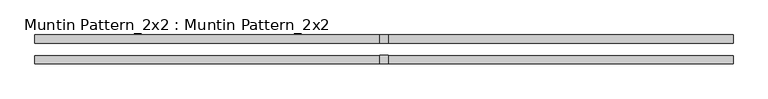
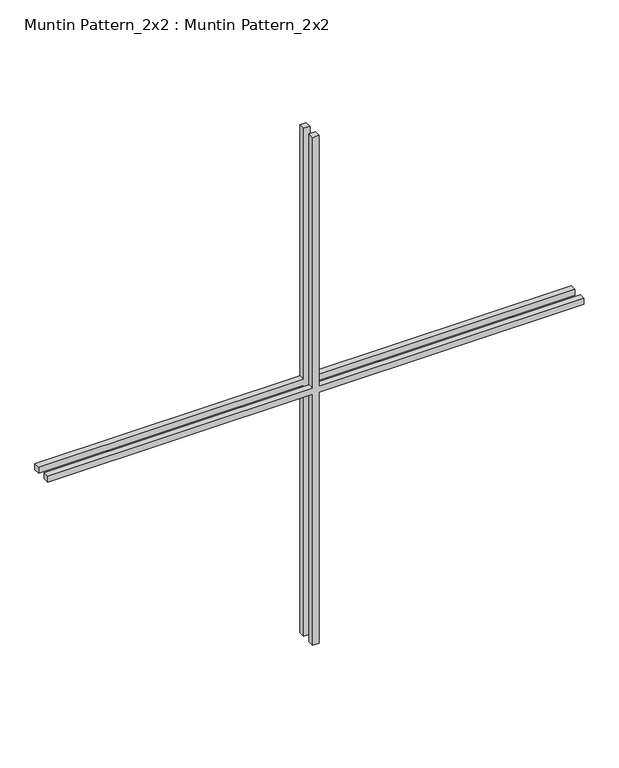
"""IFC4 building model written with IfcOpenShell, lengths in millimetres: proxy geometry, Muntin Pattern_2x2 : Muntin Pattern_2x2."""

from ifc_helpers import new_model, si_unit, frame, origin, place, context, project, spatial, polyline, outline, extrude, source, transform, mapped, element, save


def muntin_pattern_2x2_muntin_pattern_2x2_8235f178(model_context):
    return source(origin(), model_context, "Body", "SweptSolid", [
        extrude(outline(polyline([(546.1, -6.35), (546.1, -539.75), (533.4, -539.75), (533.4, -6.35), (0.0, -6.35), (0.0, 6.35), (533.4, 6.35), (533.4, 539.75), (546.1, 539.75), (546.1, 6.35), (1079.5, 6.35), (1079.5, -6.35), (546.1, -6.35)])), frame((0.0, 9.525, 0.0), z_axis=(0.0, 1.0, 0.0), x_axis=(0.0, 0.0, 1.0)), (0.0, 0.0, 1.0), 12.7),
        extrude(outline(polyline([(546.1, -6.35), (546.1, -539.75), (533.4, -539.75), (533.4, -6.35), (0.0, -6.35), (0.0, 6.35), (533.4, 6.35), (533.4, 539.75), (546.1, 539.75), (546.1, 6.35), (1079.5, 6.35), (1079.5, -6.35), (546.1, -6.35)])), frame((0.0, -22.225, 0.0), z_axis=(0.0, 1.0, 0.0), x_axis=(0.0, 0.0, 1.0)), (0.0, 0.0, 1.0), 12.7),
    ])


if __name__ == "__main__":
    model = new_model("IFC4")
    model_context = context("Model", 3, world=origin())
    ifc_project = project(units=[si_unit("LENGTHUNIT", "METRE", prefix="MILLI")], contexts=[model_context])
    site = spatial("IfcSite", under=ifc_project)
    building = spatial("IfcBuilding", under=site)
    placement = place(None, origin())
    muntin_pattern_2x2_muntin_pattern_2x2_shape = muntin_pattern_2x2_muntin_pattern_2x2_8235f178(model_context)
    element("IfcBuildingElementProxy", 1, Name="Muntin Pattern_2x2 : Muntin Pattern_2x2", ObjectType="Muntin Pattern_2x2 : Muntin Pattern_2x2", at=placement, inside=building, context=model_context, shape_type="MappedRepresentation", body=[
        mapped(muntin_pattern_2x2_muntin_pattern_2x2_shape, transform((0.0, 0.0, 0.0), x_axis=(1.0, 0.0, 0.0), y_axis=(0.0, 1.0, 0.0), z_axis=(0.0, 0.0, 1.0))),
    ])
    save(model, "model.ifc")

# Revit data of these elements
# Type "Muntin Pattern_2x2 : Muntin Pattern_2x2"
#   Width [instance default] = 4' - 0"
#   Thickness = 0' - 0 1/2"
#   Height [instance default] = 4' - 0"
#   Distance = 0' - 0 3/4"
#   Interior Material [instance default] = none
#   Exterior Material [instance default] = none
#   Default Elevation = 0
# Element 1 (IfcBuildingElementProxy, "Muntin Pattern_2x2 : Muntin Pattern_2x2")
#   Width = 3' - 6 1/2"
#   Height = 3' - 6 1/2"
#   Interior Material = Wood - Stained
#   Exterior Material = Clad - White
#   Materials on its faces: "Clad - White", "Wood - Stained"
# Materials
#   "Clad - White": class "Wood", colour RGB 242 242 238, transparency 0, Cost = 0
#   "Wood - Stained": class "Wood", colour RGB 224 178 126, transparency 0, Cost = 0
